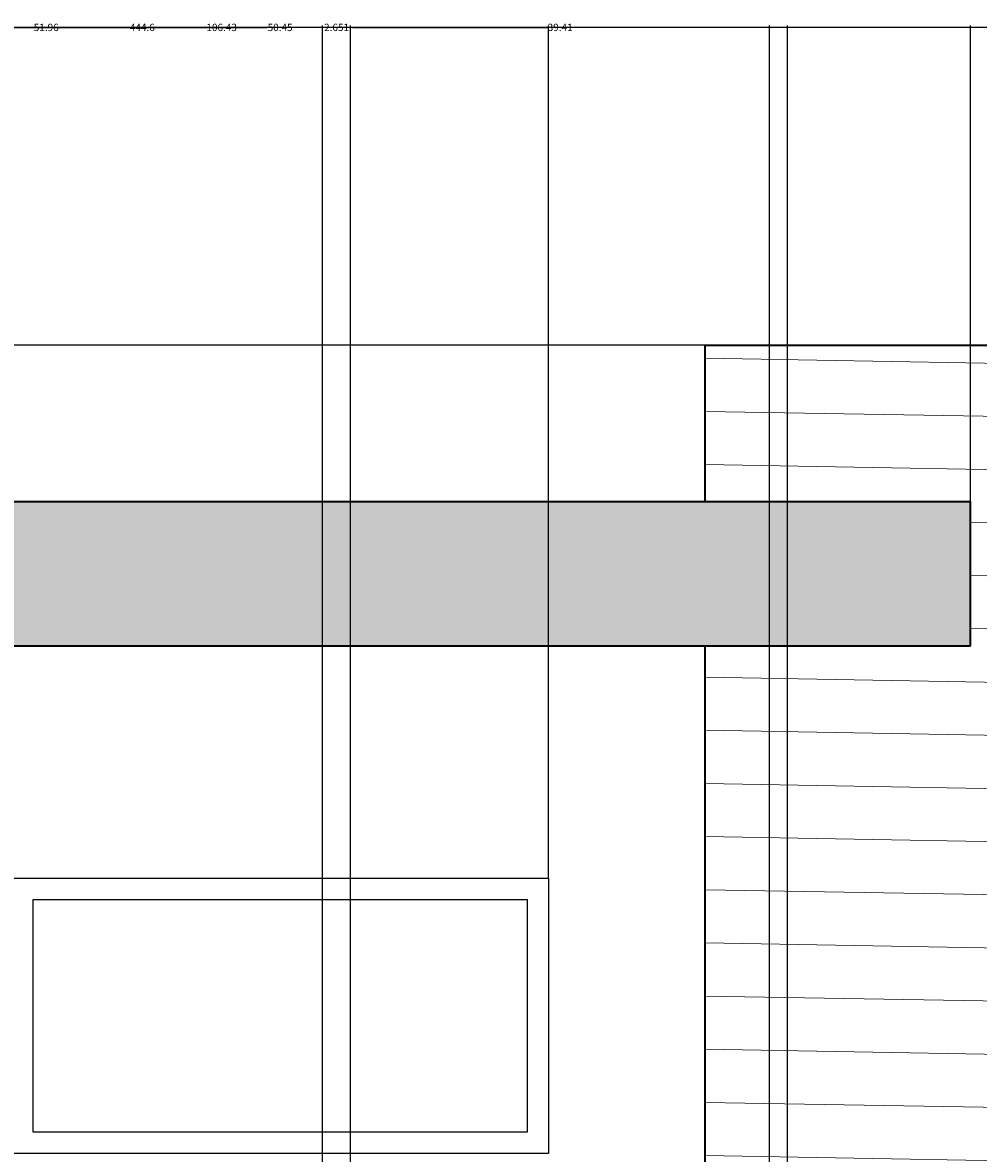
# Model space of a CAD drawing. Units: inches. Extents: x -145 to 510, y 5 to 386.
# Tile 22 of 25: x 245 to 335, y 280 to 386. Entities that reach past the tile are written whole.
import ezdxf

# ---------------------------------------------------------------- set-up
doc = ezdxf.new("R2010")
doc.units = ezdxf.units.IN
doc.header["$MEASUREMENT"] = 0
for name, color, linetype, lineweight in [('A-ANNO-DIMS', 2, 'Continuous', 18), ('A-ELEV', 7, 'Continuous', 35), ('A-ELEV-PATT', 8, 'Continuous', 13), ('A-GLAZ', 4, 'Continuous', 25)]:
    doc.layers.add(name, color=color, linetype=linetype, lineweight=lineweight)
doc.styles.get("Standard").update_dxf_attribs({"font": 'arial.ttf'})
doc.dimstyles.get("Standard").update_dxf_attribs({"dimtxt": 0.6875, "dimasz": 0.18, "dimexe": 0.18, "dimexo": 0.0625, "dimgap": 0.09, "dimtad": 0, "dimtih": 1, "dimtoh": 1, "dimdec": 4, "dimzin": 0, "dimdsep": 46, "dimlunit": 4, "dimtxsty": 'Standard', "dimcen": 0.09, "dimadec": 0, "dimazin": 0, "dimtfac": 1, "dimtdec": 4, "dimtofl": 0, "dimtmove": 0, "dimatfit": 3, "dimfxl": 1, "dimtolj": 1, "dimtzin": 0, "dimarcsym": 0})

# ---------------------------------------------------------------- blocks, each defined once
blk = doc.blocks.new('*D14')
at = {"layer": 'A-ANNO-DIMS', "color": 0, "lineweight": -2, "transparency": 16777216}
for p, q in [((34.27, 341.23), (34.27, 385.97)), ((34.45, 385.79), (255.28, 385.79)), ((478.65, 385.79), (257.81, 385.79)), ((478.83, 355.95), (478.83, 385.97))]:
    blk.add_line(p, q, dxfattribs=at)
at = {"layer": 'A-ANNO-DIMS', "color": 0, "transparency": 16777216}
for points in [[(34.45, 385.82), (34.45, 385.76), (34.27, 385.79)], [(478.65, 385.82), (478.65, 385.76), (478.83, 385.79)]]:
    blk.add_solid(points, dxfattribs=at)
at = {"layer": 'Defpoints', "color": 0, "transparency": 16777216}
for p in [(478.83, 385.79), (478.83, 355.89), (34.27, 341.17)]:
    blk.add_point(p, dxfattribs=at)
at = {"layer": 'A-ANNO-DIMS', "color": 0, "transparency": 16777216, "insert": (256.55, 385.79), "char_height": 0.688, "attachment_point": 5}
blk.add_mtext('\\A1;444.6', dxfattribs=at)
blk = doc.blocks.new('*D18')
at = {"layer": 'A-ANNO-DIMS', "color": 0, "lineweight": -2, "transparency": 16777216}
for p, q in [((244.29, 305.8), (244.29, 385.97)), ((244.47, 385.79), (268.26, 385.79)), ((294.56, 385.79), (270.77, 385.79)), ((294.74, 305.8), (294.74, 385.97))]:
    blk.add_line(p, q, dxfattribs=at)
at = {"layer": 'A-ANNO-DIMS', "color": 0, "transparency": 16777216}
for points in [[(244.47, 385.82), (244.47, 385.76), (244.29, 385.79)], [(294.56, 385.82), (294.56, 385.76), (294.74, 385.79)]]:
    blk.add_solid(points, dxfattribs=at)
at = {"layer": 'Defpoints', "color": 0, "transparency": 16777216}
for p in [(294.74, 385.79), (244.29, 305.74), (294.74, 305.74)]:
    blk.add_point(p, dxfattribs=at)
at = {"layer": 'A-ANNO-DIMS', "color": 0, "transparency": 16777216, "insert": (269.51, 385.79), "char_height": 0.688, "attachment_point": 5}
blk.add_mtext('\\A1;50.45', dxfattribs=at)
blk = doc.blocks.new('*D19')
at = {"layer": 'A-ANNO-DIMS', "color": 0, "lineweight": -2, "transparency": 16777216}
for p, q in [((478.76, 355.89), (-144.05, 355.89)), ((-143.87, 355.71), (-143.87, 218.33)), ((-143.87, 80.07), (-143.87, 217.45)), ((-114.04, 79.89), (-144.05, 79.89))]:
    blk.add_line(p, q, dxfattribs=at)
at = {"layer": 'A-ANNO-DIMS', "color": 0, "transparency": 16777216}
for points in [[(-143.9, 355.71), (-143.84, 355.71), (-143.87, 355.89)], [(-143.9, 80.07), (-143.84, 80.07), (-143.87, 79.89)]]:
    blk.add_solid(points, dxfattribs=at)
at = {"layer": 'Defpoints', "color": 0, "transparency": 16777216}
for p in [(-143.87, 355.89), (478.83, 355.89), (-113.97, 79.89)]:
    blk.add_point(p, dxfattribs=at)
at = {"layer": 'A-ANNO-DIMS', "color": 0, "transparency": 16777216, "insert": (-143.87, 217.89), "char_height": 0.688, "attachment_point": 5}
blk.add_mtext('\\A1;276', dxfattribs=at)
blk = doc.blocks.new('*D43')
at = {"layer": 'A-ANNO-DIMS', "color": 0, "lineweight": -2, "transparency": 16777216}
for p, q in [((34.27, 341.23), (34.27, 385.97)), ((34.45, 385.79), (182.84, 385.79)), ((334.26, 385.79), (185.87, 385.79)), ((334.44, 327.67), (334.44, 385.97))]:
    blk.add_line(p, q, dxfattribs=at)
at = {"layer": 'A-ANNO-DIMS', "color": 0, "transparency": 16777216}
for points in [[(34.45, 385.82), (34.45, 385.76), (34.27, 385.79)], [(334.26, 385.82), (334.26, 385.76), (334.44, 385.79)]]:
    blk.add_solid(points, dxfattribs=at)
at = {"layer": 'Defpoints', "color": 0, "transparency": 16777216}
for p in [(334.44, 385.79), (34.27, 341.17), (334.44, 327.61)]:
    blk.add_point(p, dxfattribs=at)
at = {"layer": 'A-ANNO-DIMS', "color": 0, "transparency": 16777216, "insert": (184.36, 385.79), "char_height": 0.688, "attachment_point": 5}
blk.add_mtext('\\A1;300.17', dxfattribs=at)
blk = doc.blocks.new('*D45')
at = {"layer": 'A-ANNO-DIMS', "color": 0, "lineweight": -2, "transparency": 16777216}
for p, q in [((210.8, 188.37), (210.8, 385.97)), ((210.98, 385.79), (262.53, 385.79)), ((317.05, 385.79), (265.5, 385.79)), ((317.23, 178.08), (317.23, 385.97))]:
    blk.add_line(p, q, dxfattribs=at)
at = {"layer": 'A-ANNO-DIMS', "color": 0, "transparency": 16777216}
for points in [[(210.98, 385.82), (210.98, 385.76), (210.8, 385.79)], [(317.05, 385.82), (317.05, 385.76), (317.23, 385.79)]]:
    blk.add_solid(points, dxfattribs=at)
at = {"layer": 'Defpoints', "color": 0, "transparency": 16777216}
for p in [(317.23, 385.79), (210.8, 188.31), (317.23, 178.02)]:
    blk.add_point(p, dxfattribs=at)
at = {"layer": 'A-ANNO-DIMS', "color": 0, "transparency": 16777216, "insert": (264.01, 385.79), "char_height": 0.688, "attachment_point": 5}
blk.add_mtext('\\A1;106.43', dxfattribs=at)
blk = doc.blocks.new('*D50')
at = {"layer": 'A-ANNO-DIMS', "color": 0, "lineweight": -2, "transparency": 16777216}
for p, q in [((221.53, 156.67), (221.53, 385.97)), ((221.71, 385.79), (246.26, 385.79)), ((273.31, 385.79), (248.76, 385.79)), ((273.49, 156.67), (273.49, 385.97))]:
    blk.add_line(p, q, dxfattribs=at)
at = {"layer": 'A-ANNO-DIMS', "color": 0, "transparency": 16777216}
for points in [[(221.71, 385.82), (221.71, 385.76), (221.53, 385.79)], [(273.31, 385.82), (273.31, 385.76), (273.49, 385.79)]]:
    blk.add_solid(points, dxfattribs=at)
at = {"layer": 'Defpoints', "color": 0, "transparency": 16777216}
for p in [(273.49, 385.79), (221.53, 156.61), (273.49, 156.61)]:
    blk.add_point(p, dxfattribs=at)
at = {"layer": 'A-ANNO-DIMS', "color": 0, "transparency": 16777216, "insert": (247.51, 385.79), "char_height": 0.688, "attachment_point": 5}
blk.add_mtext('\\A1;51.96', dxfattribs=at)
blk = doc.blocks.new('*D51')
at = {"layer": 'A-ANNO-DIMS', "color": 0, "lineweight": -2, "transparency": 16777216}
for p, q in [((273.31, 385.79), (273.13, 385.79)), ((273.49, 156.67), (273.49, 385.97)), ((276.14, 156.67), (276.14, 385.97)), ((276.32, 385.79), (276.5, 385.79))]:
    blk.add_line(p, q, dxfattribs=at)
at = {"layer": 'A-ANNO-DIMS', "color": 0, "transparency": 16777216}
for points in [[(273.31, 385.82), (273.31, 385.76), (273.49, 385.79)], [(276.32, 385.82), (276.32, 385.76), (276.14, 385.79)]]:
    blk.add_solid(points, dxfattribs=at)
at = {"layer": 'Defpoints', "color": 0, "transparency": 16777216}
for p in [(276.14, 385.79), (273.49, 156.61), (276.14, 156.61)]:
    blk.add_point(p, dxfattribs=at)
at = {"layer": 'A-ANNO-DIMS', "color": 0, "transparency": 16777216, "insert": (274.82, 385.79), "char_height": 0.688, "attachment_point": 5}
blk.add_mtext('\\A1;2.651', dxfattribs=at)
blk = doc.blocks.new('*D52')
at = {"layer": 'A-ANNO-DIMS', "color": 0, "lineweight": -2, "transparency": 16777216}
for p, q in [((276.14, 156.67), (276.14, 385.97)), ((276.32, 385.79), (294.66, 385.79)), ((315.37, 385.79), (297.03, 385.79)), ((315.55, 156.67), (315.55, 385.97))]:
    blk.add_line(p, q, dxfattribs=at)
at = {"layer": 'A-ANNO-DIMS', "color": 0, "transparency": 16777216}
for points in [[(276.32, 385.82), (276.32, 385.76), (276.14, 385.79)], [(315.37, 385.82), (315.37, 385.76), (315.55, 385.79)]]:
    blk.add_solid(points, dxfattribs=at)
at = {"layer": 'Defpoints', "color": 0, "transparency": 16777216}
for p in [(315.55, 385.79), (276.14, 156.61), (315.55, 156.61)]:
    blk.add_point(p, dxfattribs=at)
at = {"layer": 'A-ANNO-DIMS', "color": 0, "transparency": 16777216, "insert": (295.85, 385.79), "char_height": 0.688, "attachment_point": 5}
blk.add_mtext('\\A1;39.41', dxfattribs=at)

msp = doc.modelspace()

# ---------------------------------------------------------------- hatches: boundary and pattern name
at = {"layer": 'A-ELEV-PATT'}
h = msp.add_hatch(dxfattribs=at)
h.set_pattern_fill('ANSI31', color=256, scale=40, angle=134)
h.paths.add_polyline_path([(478.8263, 355.8905), (309.4739, 355.8905), (309.4739, 341.168), (334.4402, 341.168), (334.4402, 327.6093), (309.4739, 327.6093), (309.4739, 271.8905), (478.8263, 271.8905)])
h.paths.add_polyline_path([(442.9009, 301.8821), (351.234, 301.8821), (351.234, 332.4358), (442.9009, 332.4358)], flags=16)
h.paths.add_polyline_path([(440.9009, 303.8821), (353.234, 303.8821), (353.234, 330.4358), (440.9009, 330.4358)], flags=0)
h = msp.add_hatch(color=256, dxfattribs=at)
h.dxf.hatch_style = 1
h.paths.add_polyline_path([(334.4402, 341.168), (69.7763, 341.168), (69.7763, 327.6093), (334.4402, 327.6093)])
h.paths.add_polyline_path([(69.7763, 341.168), (34.2706, 341.168), (34.2706, 327.6093), (69.7763, 327.6093)])
h.paths.add_polyline_path([(317.2273, 188.3087), (210.7973, 188.3087), (210.7973, 178.0195), (317.2273, 178.0195)])
h.paths.add_polyline_path([(474.4893, 235.8905), (317.2273, 235.8905), (317.2273, 223.8905), (474.4893, 223.8905)])
h.paths.add_polyline_path([(317.2273, 235.8905), (309.4739, 235.8905), (309.4739, 223.8905), (317.2273, 223.8905)])
h.paths.add_polyline_path([(478.8263, 235.8905), (474.4893, 235.8905), (474.4893, 223.8905), (478.8263, 223.8905)])

# ---------------------------------------------------------------- linework, layer by layer
at = {"layer": 'A-ELEV'}
for p, q in [((309.4739, 355.8905), (478.8263, 355.8905)), ((309.4739, 341.168), (309.4739, 355.8905)), ((69.7763, 341.168), (334.4402, 341.168)), ((334.4402, 327.6093), (334.4402, 341.168)), ((34.2706, 327.6093), (334.4402, 327.6093)), ((309.4739, 271.8905), (309.4739, 327.6093))]:
    msp.add_line(p, q, dxfattribs=at)
at = {"layer": 'A-GLAZ'}
for points in [[(244.2916, 305.7416), (294.738, 305.7416), (294.738, 279.8443), (244.2916, 279.8443)], [(246.2916, 303.7416), (292.738, 303.7416), (292.738, 281.8443), (246.2916, 281.8443)]]:
    msp.add_lwpolyline(points, close=True, dxfattribs=at)

# ---------------------------------------------------------------- dimensions: what is measured, and where the dimension line sits
at = {"layer": 'A-ANNO-DIMS'}
for base, p1, p2, override, picture, middle in [((478.8263, 385.7905), (34.2706, 341.168), (478.8263, 355.8905), {"dimdec": 1, "dimlfac": 1, "dimrnd": 0, "dimzin": 0, "dimdsep": 46, "dimlunit": 2}, '*D14', (256.5484, 385.7905)), ((334.4402, 385.7905), (34.2706, 341.168), (334.4402, 327.6093), {"dimdec": 2, "dimlfac": 1, "dimrnd": 0, "dimzin": 0, "dimdsep": 46, "dimlunit": 2}, '*D43', (184.3554, 385.7905)), ((317.2273, 385.7905), (210.7973, 188.3087), (317.2273, 178.0195), {"dimdec": 2, "dimlfac": 1, "dimrnd": 0, "dimzin": 0, "dimdsep": 46, "dimlunit": 2}, '*D45', (264.0123, 385.7905)), ((273.4905, 385.7905), (221.5292, 156.6093), (273.4905, 156.6093), {"dimdec": 2, "dimlfac": 1, "dimrnd": 0, "dimzin": 0, "dimdsep": 46, "dimlunit": 2}, '*D50', (247.5098, 385.7905)), ((294.738, 385.7905), (244.2916, 305.7416), (294.738, 305.7416), {"dimdec": 2, "dimlfac": 1, "dimrnd": 0, "dimzin": 0, "dimdsep": 46, "dimlunit": 2}, '*D18', (269.5148, 385.7905)), ((276.1416, 385.7905), (273.4905, 156.6093), (276.1416, 156.6093), {"dimdec": 3, "dimlfac": 1, "dimrnd": 0, "dimzin": 0, "dimdsep": 46, "dimlunit": 2}, '*D51', (274.8161, 385.7905)), ((315.5545, 385.7905), (276.1416, 156.6093), (315.5545, 156.6093), {"dimdec": 2, "dimlfac": 1, "dimrnd": 0, "dimzin": 0, "dimdsep": 46, "dimlunit": 2}, '*D52', (295.848, 385.7905))]:
    dim = msp.add_linear_dim(base=base, p1=p1, p2=p2, dimstyle='Standard', override=override, dxfattribs=at)
    dim.commit()
    dim.dimension.update_dxf_attribs({"geometry": picture, "text_midpoint": middle})
dim = msp.add_linear_dim(base=(-143.8737, 355.8905), p1=(-113.9737, 79.8905), p2=(478.8263, 355.8905), angle=90, dimstyle='Standard', override={"dimdec": 0, "dimlfac": 1, "dimrnd": 0, "dimzin": 0, "dimdsep": 46, "dimlunit": 2}, dxfattribs=at)
dim.commit()
dim.dimension.update_dxf_attribs({"geometry": '*D19', "text_midpoint": (-143.8737, 217.8905)})

doc.saveas('drawing.dxf')
